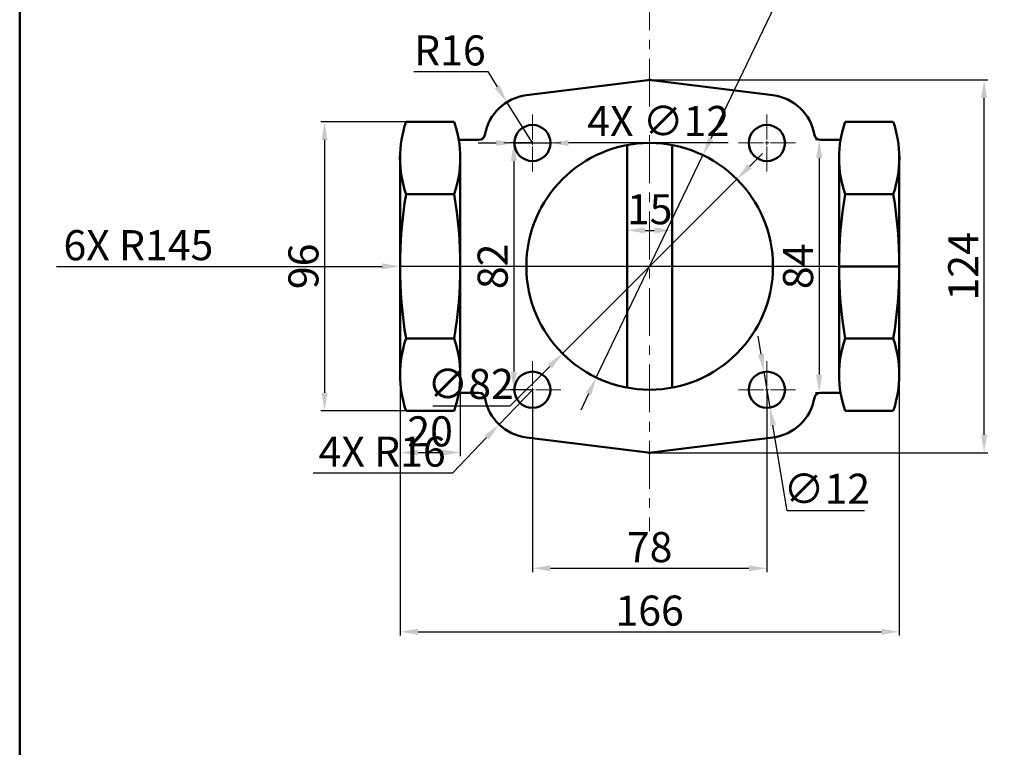
# Model space of a CAD drawing. Units: millimetres. Extents: x 147 to 984, y -369 to 435.
# Tile 4 of 10: x 147 to 475, y -48 to 193. Entities that reach past the tile are written whole.
import ezdxf

# ---------------------------------------------------------------- set-up
doc = ezdxf.new("R2010")
doc.units = ezdxf.units.MM
doc.header["$LTSCALE"] = 0.5
doc.linetypes.add('CENTER', pattern=[50.8, 31.75, -6.35, 6.35, -6.35])
for name, color, linetype, lineweight in [('M-CNTR', 1, 'CENTER', 18), ('M-DIMS', 2, 'Continuous', 25), ('M-OUTL', 7, 'Continuous', 50)]:
    doc.layers.add(name, color=color, linetype=linetype, lineweight=lineweight)
doc.styles.get("Standard").update_dxf_attribs({"font": 'arial.ttf'})
doc.dimstyles.new('ISO-25', dxfattribs={"dimtxt": 10, "dimasz": 6, "dimexe": 1.25, "dimexo": 0.625, "dimtad": 1, "dimtoh": 1, "dimdec": 0, "dimtxsty": 'Standard', "dimcen": 2.5, "dimadec": 0, "dimazin": 0, "dimtfac": 1, "dimtdec": 0, "dimtmove": 0, "dimatfit": 3, "dimfxl": 1, "dimarcsym": 0})

# ---------------------------------------------------------------- blocks, each defined once
blk = doc.blocks.new('*U12')
at = {"layer": 'M-CNTR', "color": 0, "transparency": 16777216}
for p, q in [((0, 1.2), (0, 9.5)), ((-9.5, 0), (-1.2, 0)), ((1.2, 0), (9.5, 0)), ((0, -9.5), (0, -1.2))]:
    blk.add_line(p, q, dxfattribs=at)
at = {"layer": 'M-CNTR', "color": 0, "linetype": 'Continuous', "transparency": 16777216}
for p, q in [((-0.6, 0), (0.6, 0)), ((0, -0.6), (0, 0.6))]:
    blk.add_line(p, q, dxfattribs=at)
blk = doc.blocks.new('*U13')
at = {"layer": 'M-CNTR', "color": 0, "transparency": 16777216}
for p, q in [((0, 1.2), (0, 9.5)), ((-9.5, 0), (-1.2, 0)), ((1.2, 0), (9.5, 0)), ((0, -9.5), (0, -1.2))]:
    blk.add_line(p, q, dxfattribs=at)
at = {"layer": 'M-CNTR', "color": 0, "linetype": 'Continuous', "transparency": 16777216}
for p, q in [((-0.6, 0), (0.6, 0)), ((0, -0.6), (0, 0.6))]:
    blk.add_line(p, q, dxfattribs=at)
blk = doc.blocks.new('*U14')
at = {"layer": 'M-CNTR', "color": 0, "transparency": 16777216}
for p, q in [((0, 1.2), (0, 9.5)), ((-9.5, 0), (-1.2, 0)), ((1.2, 0), (9.5, 0)), ((0, -9.5), (0, -1.2))]:
    blk.add_line(p, q, dxfattribs=at)
at = {"layer": 'M-CNTR', "color": 0, "linetype": 'Continuous', "transparency": 16777216}
for p, q in [((-0.6, 0), (0.6, 0)), ((0, -0.6), (0, 0.6))]:
    blk.add_line(p, q, dxfattribs=at)
blk = doc.blocks.new('*U15')
at = {"layer": 'M-CNTR', "color": 0, "transparency": 16777216}
for p, q in [((0, 1.2), (0, 9.5)), ((-9.5, 0), (-1.2, 0)), ((1.2, 0), (9.5, 0)), ((0, -9.5), (0, -1.2))]:
    blk.add_line(p, q, dxfattribs=at)
at = {"layer": 'M-CNTR', "color": 0, "linetype": 'Continuous', "transparency": 16777216}
for p, q in [((-0.6, 0), (0.6, 0)), ((0, -0.6), (0, 0.6))]:
    blk.add_line(p, q, dxfattribs=at)
blk = doc.blocks.new('*D16')
at = {"layer": 'Defpoints', "color": 0, "transparency": 16777216}
for p in [(349.32, 127.06), (364.32, 127.06), (364.32, 123.48)]:
    blk.add_point(p, dxfattribs=at)
at = {"layer": 'M-DIMS', "color": 0, "lineweight": -2, "transparency": 16777216}
for p, q in [((349.32, 126.44), (349.32, 122.23)), ((364.32, 126.44), (364.32, 122.23)), ((355.32, 123.48), (358.32, 123.48))]:
    blk.add_line(p, q, dxfattribs=at)
at = {"layer": 'M-DIMS', "color": 0, "transparency": 16777216}
for points in [[(355.32, 124.48), (355.32, 122.48), (349.32, 123.48)], [(358.32, 124.48), (358.32, 122.48), (364.32, 123.48)]]:
    blk.add_solid(points, dxfattribs=at)
at = {"layer": 'M-DIMS', "color": 0, "transparency": 16777216, "insert": (356.82, 129.21), "char_height": 10, "attachment_point": 5}
blk.add_mtext('15', dxfattribs=at)
blk = doc.blocks.new('*D17')
at = {"layer": 'Defpoints', "color": 0, "transparency": 16777216}
for p in [(283.82, 159.52), (248.72, 63.52), (283.82, 63.52)]:
    blk.add_point(p, dxfattribs=at)
at = {"layer": 'M-DIMS', "color": 0, "lineweight": -2, "transparency": 16777216}
for p, q in [((283.19, 159.52), (247.47, 159.52)), ((248.72, 153.52), (248.72, 69.52)), ((283.19, 63.52), (247.47, 63.52))]:
    blk.add_line(p, q, dxfattribs=at)
at = {"layer": 'M-DIMS', "color": 0, "transparency": 16777216}
for points in [[(247.72, 153.52), (249.72, 153.52), (248.72, 159.52)], [(247.72, 69.52), (249.72, 69.52), (248.72, 63.52)]]:
    blk.add_solid(points, dxfattribs=at)
at = {"layer": 'M-DIMS', "color": 0, "transparency": 16777216, "insert": (242.99, 111.52), "char_height": 10, "attachment_point": 5, "rotation": 90}
blk.add_mtext('96', dxfattribs=at)
blk = doc.blocks.new('*D18')
at = {"layer": 'Defpoints', "color": 0, "transparency": 16777216}
for p in [(356.82, 173.48), (468.02, 173.48), (356.82, 49.56)]:
    blk.add_point(p, dxfattribs=at)
at = {"layer": 'M-DIMS', "color": 0, "lineweight": -2, "transparency": 16777216}
for p, q in [((357.44, 173.48), (469.27, 173.48)), ((468.02, 55.56), (468.02, 167.48)), ((357.44, 49.56), (469.27, 49.56))]:
    blk.add_line(p, q, dxfattribs=at)
at = {"layer": 'M-DIMS', "color": 0, "transparency": 16777216}
for points in [[(467.02, 167.48), (469.02, 167.48), (468.02, 173.48)], [(467.02, 55.56), (469.02, 55.56), (468.02, 49.56)]]:
    blk.add_solid(points, dxfattribs=at)
at = {"layer": 'M-DIMS', "color": 0, "transparency": 16777216, "insert": (462.38, 111.52), "char_height": 10, "attachment_point": 5, "rotation": 90}
blk.add_mtext('124', dxfattribs=at)
blk = doc.blocks.new('*D19')
at = {"layer": 'Defpoints', "color": 0, "transparency": 16777216}
for p in [(309.33, 166.08), (317.82, 152.52)]:
    blk.add_point(p, dxfattribs=at)
at = {"layer": 'M-DIMS', "color": 0, "lineweight": -2, "transparency": 16777216}
for p, q in [((278.45, 176.25), (302.97, 176.25)), ((302.97, 176.25), (306.15, 171.17)), ((317.82, 152.52), (309.33, 166.08))]:
    blk.add_line(p, q, dxfattribs=at)
at = {"layer": 'M-DIMS', "color": 0, "transparency": 16777216}
blk.add_solid([(307, 171.7), (305.3, 170.64), (309.33, 166.08)], dxfattribs=at)
at = {"layer": 'M-DIMS', "color": 0, "transparency": 16777216, "insert": (290.4, 181.99), "char_height": 10, "attachment_point": 5}
blk.add_mtext('R16', dxfattribs=at)
blk = doc.blocks.new('*D20')
at = {"layer": 'Defpoints', "color": 0, "transparency": 16777216}
for p in [(394.83, 76.44), (396.81, 64.6)]:
    blk.add_point(p, dxfattribs=at)
at = {"layer": 'M-DIMS', "color": 0, "lineweight": -2, "transparency": 16777216}
for p, q in [((393.84, 82.35), (392.85, 88.27)), ((394.83, 76.44), (396.81, 64.6)), ((402.54, 30.29), (397.8, 58.68)), ((428.27, 30.29), (402.54, 30.29))]:
    blk.add_line(p, q, dxfattribs=at)
at = {"layer": 'M-DIMS', "color": 0, "transparency": 16777216}
for points in [[(394.83, 82.52), (392.85, 82.19), (394.83, 76.44)], [(398.78, 58.85), (396.81, 58.52), (396.81, 64.6)]]:
    blk.add_solid(points, dxfattribs=at)
at = {"layer": 'M-DIMS', "color": 0, "transparency": 16777216, "insert": (415.72, 36.3), "char_height": 10, "attachment_point": 5}
blk.add_mtext('∅12', dxfattribs=at)
blk = doc.blocks.new('*D21')
at = {"layer": 'Defpoints', "color": 0, "transparency": 16777216}
for p in [(293.83, 75.52), (273.82, 74.73), (293.83, 49.65)]:
    blk.add_point(p, dxfattribs=at)
at = {"layer": 'M-DIMS', "color": 0, "lineweight": -2, "transparency": 16777216}
for p, q in [((273.82, 74.1), (273.82, 48.4)), ((293.83, 74.89), (293.83, 48.4)), ((279.82, 49.65), (287.83, 49.65))]:
    blk.add_line(p, q, dxfattribs=at)
at = {"layer": 'M-DIMS', "color": 0, "transparency": 16777216}
for points in [[(279.82, 50.65), (279.82, 48.65), (273.82, 49.65)], [(287.83, 50.65), (287.83, 48.65), (293.83, 49.65)]]:
    blk.add_solid(points, dxfattribs=at)
at = {"layer": 'M-DIMS', "color": 0, "transparency": 16777216, "insert": (283.82, 55.38), "char_height": 10, "attachment_point": 5}
blk.add_mtext('20', dxfattribs=at)
blk = doc.blocks.new('*D22')
at = {"layer": 'Defpoints', "color": 0, "transparency": 16777216}
for p in [(273.82, 111.52), (439.82, 111.52), (439.82, -9.93)]:
    blk.add_point(p, dxfattribs=at)
at = {"layer": 'M-DIMS', "color": 0, "lineweight": -2, "transparency": 16777216}
for p, q in [((273.82, 110.89), (273.82, -11.18)), ((439.82, 110.89), (439.82, -11.18)), ((279.82, -9.93), (433.82, -9.93))]:
    blk.add_line(p, q, dxfattribs=at)
at = {"layer": 'M-DIMS', "color": 0, "transparency": 16777216}
for points in [[(279.82, -8.93), (279.82, -10.93), (273.82, -9.93)], [(433.82, -8.93), (433.82, -10.93), (439.82, -9.93)]]:
    blk.add_solid(points, dxfattribs=at)
at = {"layer": 'M-DIMS', "color": 0, "transparency": 16777216, "insert": (356.82, -4.2), "char_height": 10, "attachment_point": 5}
blk.add_mtext('166', dxfattribs=at)
blk = doc.blocks.new('*D23')
at = {"layer": 'Defpoints', "color": 0, "transparency": 16777216}
for p in [(317.82, 70.52), (395.82, 70.52), (395.82, 11.17)]:
    blk.add_point(p, dxfattribs=at)
at = {"layer": 'M-DIMS', "color": 0, "lineweight": -2, "transparency": 16777216}
for p, q in [((317.82, 69.89), (317.82, 9.92)), ((395.82, 69.89), (395.82, 9.92)), ((323.82, 11.17), (389.82, 11.17))]:
    blk.add_line(p, q, dxfattribs=at)
at = {"layer": 'M-DIMS', "color": 0, "transparency": 16777216}
for points in [[(323.82, 12.17), (323.82, 10.17), (317.82, 11.17)], [(389.82, 12.17), (389.82, 10.17), (395.82, 11.17)]]:
    blk.add_solid(points, dxfattribs=at)
at = {"layer": 'M-DIMS', "color": 0, "transparency": 16777216, "insert": (356.82, 16.9), "char_height": 10, "attachment_point": 5}
blk.add_mtext('78', dxfattribs=at)
blk = doc.blocks.new('*D24')
at = {"layer": 'Defpoints', "color": 0, "transparency": 16777216}
for p in [(416.93, 153.52), (413.18, 69.52), (416.93, 69.52)]:
    blk.add_point(p, dxfattribs=at)
at = {"layer": 'M-DIMS', "color": 0, "lineweight": -2, "transparency": 16777216}
for p, q in [((416.3, 153.52), (411.93, 153.52)), ((413.18, 147.52), (413.18, 75.52)), ((416.3, 69.52), (411.93, 69.52))]:
    blk.add_line(p, q, dxfattribs=at)
at = {"layer": 'M-DIMS', "color": 0, "transparency": 16777216}
for points in [[(412.18, 147.52), (414.18, 147.52), (413.18, 153.52)], [(412.18, 75.52), (414.18, 75.52), (413.18, 69.52)]]:
    blk.add_solid(points, dxfattribs=at)
at = {"layer": 'M-DIMS', "color": 0, "transparency": 16777216, "insert": (407.45, 111.52), "char_height": 10, "attachment_point": 5, "rotation": 90}
blk.add_mtext('84', dxfattribs=at)
blk = doc.blocks.new('*D25')
at = {"layer": 'Defpoints', "color": 0, "transparency": 16777216}
for p in [(317.82, 152.52), (311.65, 70.52), (317.82, 70.52)]:
    blk.add_point(p, dxfattribs=at)
at = {"layer": 'M-DIMS', "color": 0, "lineweight": -2, "transparency": 16777216}
for p, q in [((317.19, 152.52), (310.4, 152.52)), ((311.65, 146.52), (311.65, 76.52)), ((317.19, 70.52), (310.4, 70.52))]:
    blk.add_line(p, q, dxfattribs=at)
at = {"layer": 'M-DIMS', "color": 0, "transparency": 16777216}
for points in [[(310.65, 146.52), (312.65, 146.52), (311.65, 152.52)], [(310.65, 76.52), (312.65, 76.52), (311.65, 70.52)]]:
    blk.add_solid(points, dxfattribs=at)
at = {"layer": 'M-DIMS', "color": 0, "transparency": 16777216, "insert": (305.91, 111.52), "char_height": 10, "attachment_point": 5, "rotation": 90}
blk.add_mtext('82', dxfattribs=at)
blk = doc.blocks.new('*D26')
at = {"layer": 'Defpoints', "color": 0, "transparency": 16777216}
for p in [(374.55, 148.48), (339.08, 74.55)]:
    blk.add_point(p, dxfattribs=at)
at = {"layer": 'M-DIMS', "color": 0, "lineweight": -2, "transparency": 16777216}
for p, q in [((398.44, 198.26), (377.15, 153.89)), ((424.17, 198.26), (398.44, 198.26)), ((339.08, 74.55), (374.55, 148.48)), ((336.49, 69.14), (333.89, 63.73))]:
    blk.add_line(p, q, dxfattribs=at)
at = {"layer": 'M-DIMS', "color": 0, "transparency": 16777216}
for points in [[(376.25, 154.33), (378.05, 153.46), (374.55, 148.48)], [(335.58, 69.58), (337.39, 68.71), (339.08, 74.55)]]:
    blk.add_solid(points, dxfattribs=at)
at = {"layer": 'M-DIMS', "color": 0, "transparency": 16777216, "insert": (411.62, 204.27), "char_height": 10, "attachment_point": 5}
blk.add_mtext('∅82', dxfattribs=at)
blk = doc.blocks.new('*D157')
at = {"layer": 'Defpoints', "color": 0, "ltscale": 0.5, "transparency": 16777216}
for p in [(317.82, 70.52), (306.75, 58.96)]:
    blk.add_point(p, dxfattribs=at)
at = {"layer": 'M-DIMS', "color": 0, "lineweight": -2, "ltscale": 0.5, "transparency": 16777216}
for p, q in [((317.82, 70.52), (306.75, 58.96)), ((291.39, 42.92), (302.6, 54.63)), ((244.98, 42.92), (291.39, 42.92))]:
    blk.add_line(p, q, dxfattribs=at)
at = {"layer": 'M-DIMS', "color": 0, "ltscale": 0.5, "transparency": 16777216}
blk.add_solid([(301.88, 55.32), (303.32, 53.94), (306.75, 58.96)], dxfattribs=at)
at = {"layer": 'M-DIMS', "color": 0, "ltscale": 0.5, "transparency": 16777216, "insert": (267.87, 48.65), "char_height": 10, "attachment_point": 5}
blk.add_mtext('4X R16', dxfattribs=at)
blk = doc.blocks.new('*D158')
at = {"layer": 'Defpoints', "color": 0, "ltscale": 0.5, "transparency": 16777216}
for p in [(311.82, 152.52), (323.82, 152.52)]:
    blk.add_point(p, dxfattribs=at)
at = {"layer": 'M-DIMS', "color": 0, "lineweight": -2, "ltscale": 0.5, "transparency": 16777216}
for p, q in [((305.82, 152.51), (299.82, 152.51)), ((311.82, 152.52), (323.82, 152.52)), ((335.82, 152.52), (329.82, 152.52)), ((382.9, 152.52), (335.82, 152.52))]:
    blk.add_line(p, q, dxfattribs=at)
at = {"layer": 'M-DIMS', "color": 0, "ltscale": 0.5, "transparency": 16777216}
for points in [[(305.82, 153.51), (305.82, 151.51), (311.82, 152.52)], [(329.82, 153.52), (329.82, 151.52), (323.82, 152.52)]]:
    blk.add_solid(points, dxfattribs=at)
at = {"layer": 'M-DIMS', "color": 0, "ltscale": 0.5, "transparency": 16777216, "insert": (359.67, 158.53), "char_height": 10, "attachment_point": 5}
blk.add_mtext('4X ∅12', dxfattribs=at)
blk = doc.blocks.new('*D159')
at = {"layer": 'Defpoints', "color": 0, "ltscale": 0.5, "transparency": 16777216}
for p in [(385.81, 140.51), (327.83, 82.53)]:
    blk.add_point(p, dxfattribs=at)
at = {"layer": 'M-DIMS', "color": 0, "lineweight": -2, "ltscale": 0.5, "transparency": 16777216}
for p, q in [((390.05, 144.75), (394.29, 148.99)), ((385.81, 140.51), (327.83, 82.53)), ((310.43, 65.13), (323.58, 78.28)), ((284.7, 65.13), (310.43, 65.13))]:
    blk.add_line(p, q, dxfattribs=at)
at = {"layer": 'M-DIMS', "color": 0, "ltscale": 0.5, "transparency": 16777216}
for points in [[(389.34, 145.46), (390.76, 144.05), (385.81, 140.51)], [(322.88, 78.99), (324.29, 77.58), (327.83, 82.53)]]:
    blk.add_solid(points, dxfattribs=at)
at = {"layer": 'M-DIMS', "color": 0, "ltscale": 0.5, "transparency": 16777216, "insert": (297.26, 71.14), "char_height": 10, "attachment_point": 5}
blk.add_mtext('∅82', dxfattribs=at)
blk = doc.blocks.new('*D160')
at = {"layer": 'Defpoints', "color": 0, "ltscale": 0.5, "transparency": 16777216}
for p in [(273.82, 111.52), (418.82, 111.52)]:
    blk.add_point(p, dxfattribs=at)
at = {"layer": 'M-DIMS', "color": 0, "lineweight": -2, "ltscale": 0.5, "transparency": 16777216}
for p, q in [((159.55, 111.52), (267.82, 111.52)), ((418.82, 111.52), (273.82, 111.52))]:
    blk.add_line(p, q, dxfattribs=at)
at = {"layer": 'M-DIMS', "color": 0, "ltscale": 0.5, "transparency": 16777216}
blk.add_solid([(267.82, 112.52), (267.82, 110.52), (273.82, 111.52)], dxfattribs=at)
at = {"layer": 'M-DIMS', "color": 0, "ltscale": 0.5, "transparency": 16777216, "insert": (186.82, 117.25), "char_height": 10, "attachment_point": 5}
blk.add_mtext('6X R145', dxfattribs=at)

msp = doc.modelspace()

# ---------------------------------------------------------------- linework, layer by layer
at = {"layer": 'M-CNTR'}
for p, q in [((356.8179, 307.4916), (356.8179, 23.5276)), ((419.8179, 111.5181), (273.8179, 111.5181))]:
    msp.add_line(p, q, dxfattribs=at)
at = {"layer": 'M-OUTL'}
for p, q in [((315.8332, 168.3945), (356.1977, 173.4406)), ((357.4381, 173.4406), (397.8026, 168.3945)), ((291.8179, 159.5181), (275.8179, 159.5181)), ((437.8179, 159.5181), (421.8179, 159.5181)), ((293.345, 153.5181), (300.0697, 153.5181)), ((349.3179, 151.8263), (349.3179, 71.2099)), ((364.3179, 151.8263), (364.3179, 71.2099)), ((413.5661, 153.5181), (420.2908, 153.5181)), ((273.8179, 148.7884), (273.8179, 74.7258)), ((293.8179, 74.7258), (293.8179, 148.7884)), ((419.8179, 148.7884), (419.8179, 74.7258)), ((439.8179, 74.7258), (439.8179, 148.7884)), ((291.8179, 135.5181), (275.8179, 135.5181)), ((437.8179, 135.5181), (421.8179, 135.5181)), ((439.8179, 111.5181), (419.8179, 111.5181)), ((291.8179, 87.5181), (275.8179, 87.5181)), ((437.8179, 87.5181), (421.8179, 87.5181)), ((293.345, 69.5181), (300.0697, 69.5181)), ((413.5661, 69.5181), (420.2908, 69.5181)), ((275.8179, 63.5181), (291.8179, 63.5181)), ((421.8179, 63.5181), (437.8179, 63.5181)), ((315.8332, 54.6417), (356.1977, 49.5957)), ((357.4381, 49.5957), (397.8026, 54.6417))]:
    msp.add_line(p, q, dxfattribs=at)
at = {"layer": 'M-OUTL', "ltscale": 0.5}
msp.add_lwpolyline([(147.3511, 435.3078), (984.0884, 435.3078), (984.0884, -369.4968), (147.3511, -369.4968)], close=True, dxfattribs=at)
at = {"layer": 'M-OUTL'}
for centre, radius in [((317.8179, 152.5181), 6), ((395.8179, 152.5181), 6), ((356.8179, 111.5181), 41), ((317.8179, 70.5181), 6), ((395.8179, 70.5181), 6)]:
    msp.add_circle(centre, radius, dxfattribs=at)
for centre, radius, start, end in [((356.8179, 168.4792), 5, 82.874317, 97.125683), ((317.8179, 152.5181), 16, 97.125683, 170.405932), ((395.8179, 152.5181), 16, 9.594068, 82.874317), ((310.4145, 147.5181), 36.6187, 160.870654, 199.129346), ((257.2213, 147.5181), 36.6187, 340.870654, 19.129346), ((456.4145, 147.5181), 36.6187, 160.870654, 199.129346), ((403.2213, 147.5181), 36.6187, 340.870654, 19.129346), ((300.0697, 155.5181), 2, 270, 350.405932), ((413.5661, 155.5181), 2, 189.594068, 270), ((418.8179, 111.5181), 145, 170.472717, 189.527283), ((148.8179, 111.5181), 145, 350.472717, 9.527283), ((564.8179, 111.5181), 145, 170.472717, 189.527283), ((294.8179, 111.5181), 145, 350.472717, 9.527283), ((310.6609, 75.5181), 36.8516, 160.99621, 199.00379), ((256.9749, 75.5181), 36.8516, 340.99621, 19.00379), ((456.6609, 75.5181), 36.8516, 160.99621, 199.00379), ((402.9749, 75.5181), 36.8516, 340.99621, 19.00379), ((300.0697, 67.5181), 2, 9.594068, 90), ((413.5661, 67.5181), 2, 90, 170.405932), ((317.8179, 70.5181), 16, 189.594068, 262.874317), ((395.8179, 70.5181), 16, 277.125683, 350.405932), ((356.8179, 54.557), 5, 262.874317, 277.125683)]:
    msp.add_arc(centre, radius, start, end, dxfattribs=at)

# ---------------------------------------------------------------- block references
at = {"layer": 'M-CNTR'}
for name, p in [('*U14', (317.8179, 152.5181)), ('*U15', (395.8179, 152.5181)), ('*U13', (317.8179, 70.5181)), ('*U12', (395.8179, 70.5181))]:
    msp.add_blockref(name, p, dxfattribs=at)

# ---------------------------------------------------------------- dimensions: what is measured, and where the dimension line sits
at = {"layer": 'M-DIMS'}
for p1, p2, picture, middle in [((339.0816, 74.553), (374.5542, 148.4833), '*D26', (411.6154, 198.2633)), ((394.8285, 76.436), (396.8073, 64.6003), '*D20', (415.7202, 30.2883))]:
    dim = msp.add_diameter_dim_2p(p1=p1, p2=p2, dimstyle='ISO-25', override={"dimclrd": 0, "dimclre": 0, "dimclrt": 0}, dxfattribs=at)
    dim.commit()
    dim.dimension.update_dxf_attribs({"geometry": picture, "text_midpoint": middle, "dimtype": 163})
dim = msp.add_radius_dim(center=(317.8179, 152.5181), mpoint=(309.3314, 166.082), dimstyle='ISO-25', override={"dimclrd": 0, "dimclre": 0, "dimclrt": 0}, dxfattribs=at)
dim.commit()
dim.dimension.update_dxf_attribs({"geometry": '*D19', "text_midpoint": (290.3974, 181.9857)})
at = {"layer": 'M-DIMS', "ltscale": 0.5}
dim = msp.add_diameter_dim_2p(p1=(311.8179, 152.5163), p2=(323.8179, 152.52), text='4X <>', dimstyle='ISO-25', override={"dimdec": 0, "dimlfac": 1, "dimrnd": 0, "dimzin": 0, "dimdsep": 46, "dimlunit": 2}, dxfattribs=at)
dim.commit()
dim.dimension.update_dxf_attribs({"geometry": '*D158', "text_midpoint": (335.8179, 152.5237)})
at = {"layer": 'M-DIMS'}
for base, p1, p2, picture, middle in [((468.023, 173.4792), (356.8179, 49.557), (356.8179, 173.4792), '*D18', (462.3776, 111.5181)), ((248.7228, 63.5181), (283.8179, 159.5181), (283.8179, 63.5181), '*D17', (242.992, 111.5181)), ((311.6451, 70.5181), (317.8179, 152.5181), (317.8179, 70.5181), '*D25', (305.9144, 111.5181)), ((413.1842, 69.5181), (416.9285, 153.5181), (416.9285, 69.5181), '*D24', (407.4535, 111.5181))]:
    dim = msp.add_linear_dim(base=base, p1=p1, p2=p2, angle=90, dimstyle='ISO-25', override={"dimclrd": 0, "dimclre": 0, "dimclrt": 0}, dxfattribs=at)
    dim.commit()
    dim.dimension.update_dxf_attribs({"geometry": picture, "text_midpoint": middle})
at = {"layer": 'M-DIMS', "ltscale": 0.5}
dim = msp.add_diameter_dim_2p(p1=(385.8092, 140.5096), p2=(327.8266, 82.5266), dimstyle='ISO-25', override={"dimdec": 0, "dimlfac": 1, "dimrnd": 0, "dimzin": 0, "dimdsep": 46, "dimlunit": 2}, dxfattribs=at)
dim.commit()
dim.dimension.update_dxf_attribs({"geometry": '*D159', "text_midpoint": (297.2557, 65.1317), "dimtype": 163})
at = {"layer": 'M-DIMS'}
for base, p1, p2, picture, middle in [((364.3179, 123.4775), (349.3179, 127.0644), (364.3179, 127.0644), '*D16', (356.8179, 129.2082)), ((439.8179, -9.927), (273.8179, 111.5181), (439.8179, 111.5181), '*D22', (356.8179, -4.1963)), ((395.8179, 11.1698), (317.8179, 70.5181), (395.8179, 70.5181), '*D23', (356.8179, 16.9005))]:
    dim = msp.add_linear_dim(base=base, p1=p1, p2=p2, dimstyle='ISO-25', override={"dimclrd": 0, "dimclre": 0, "dimclrt": 0}, dxfattribs=at)
    dim.commit()
    dim.dimension.update_dxf_attribs({"geometry": picture, "text_midpoint": middle})
at = {"layer": 'M-DIMS', "ltscale": 0.5}
dim = msp.add_radius_dim(center=(418.8179, 111.5181), mpoint=(273.8179, 111.518), text='6X <>', dimstyle='ISO-25', override={"dimdec": 0, "dimlfac": 1, "dimrnd": 0, "dimzin": 0, "dimdsep": 46, "dimlunit": 2}, dxfattribs=at)
dim.commit()
dim.dimension.update_dxf_attribs({"geometry": '*D160', "text_midpoint": (186.8179, 111.518), "dimtype": 164})
at = {"layer": 'M-DIMS'}
dim = msp.add_linear_dim(base=(293.8264, 49.6486), p1=(273.8179, 74.7258), p2=(293.8264, 75.5181), dimstyle='ISO-25', override={"dimclrd": 0, "dimclre": 0, "dimclrt": 0}, dxfattribs=at)
dim.commit()
dim.dimension.update_dxf_attribs({"geometry": '*D21', "text_midpoint": (283.8222, 49.6486), "dimtype": 160})
at = {"layer": 'M-DIMS', "ltscale": 0.5}
dim = msp.add_radius_dim(center=(317.8179, 70.5181), mpoint=(306.7509, 58.9629), text='4X <>', dimstyle='ISO-25', override={"dimdec": 0, "dimlfac": 1, "dimrnd": 0, "dimzin": 0, "dimdsep": 46, "dimlunit": 2}, dxfattribs=at)
dim.commit()
dim.dimension.update_dxf_attribs({"geometry": '*D157', "text_midpoint": (267.8738, 48.6526)})

doc.saveas('drawing.dxf')
